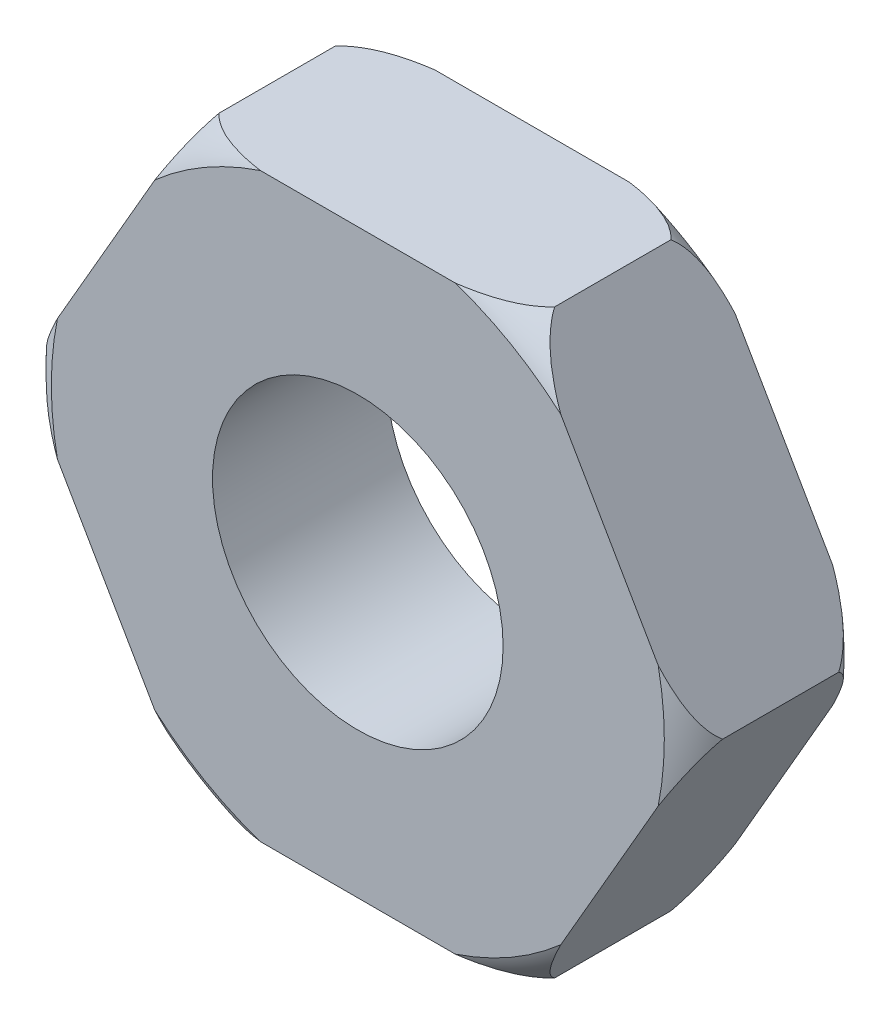
SolidWorks part; units mm, degrees
material "Plain Carbon Steel"
ref_plane "Front Plane" through (0, 0, 0) normal (0, 0, 1) x (1, 0, 0)
ref_plane "Top Plane" through (0, 0, 0) normal (0, 1, 0) x (1, 0, 0)
ref_plane "Right Plane" through (0, 0, 0) normal (1, 0, 0) x (0, 0, -1)
sketch "Hex Profile 20AF" plane through (0, 0, 0) normal (0, 0, 1) x (1, 0, 0)
  line L1 (11.547, 0) -> (5.7735, 10)
  line L2 (5.7735, 10) -> (-5.7735, 10)
  line L3 (-5.7735, 10) -> (-11.547, 0)
  line L4 (-11.547, 0) -> (-5.7735, -10)
  line L5 (-5.7735, -10) -> (5.7735, -10)
  line L6 (5.7735, -10) -> (11.547, 0)
  circle A0 centre (0, 0) radius 10 construction
  circle A1 centre (0, 0) radius 5
  dimension "D2" = 10
  dimension "D1" = 20
extrude "Hex Nut Body 6mm" add sketch "Hex Profile 20AF" along normal mid plane 6
sketch "Edge Chamfer Profile" plane through (0, 0, 0) normal (0, 1, 0) x (1, 0, 0)
  line L0 (0, 5.0769) -> (0, -7.2296) construction
  line L1 (11.547, 3) -> (5.7735, 3) construction
  line L2 (10.547, 3) -> (11.547, 3)
  line L3 (11.547, 3) -> (11.547, 2)
  arc A0 (10.547, 3) -> (11.547, 2) centre (9.7241, 1.1771) cw
  dimension "D1" = 2
  dimension "D2" = 1
  dimension "1" = 1
revolve "Edge Chamfer Cut" cut sketch "Edge Chamfer Profile" angle 360 about L0
mirror "Edge Chamfer Mirror" about plane through (0, 0, 0) normal (0, 0, 1) of "Edge Chamfer Cut"
